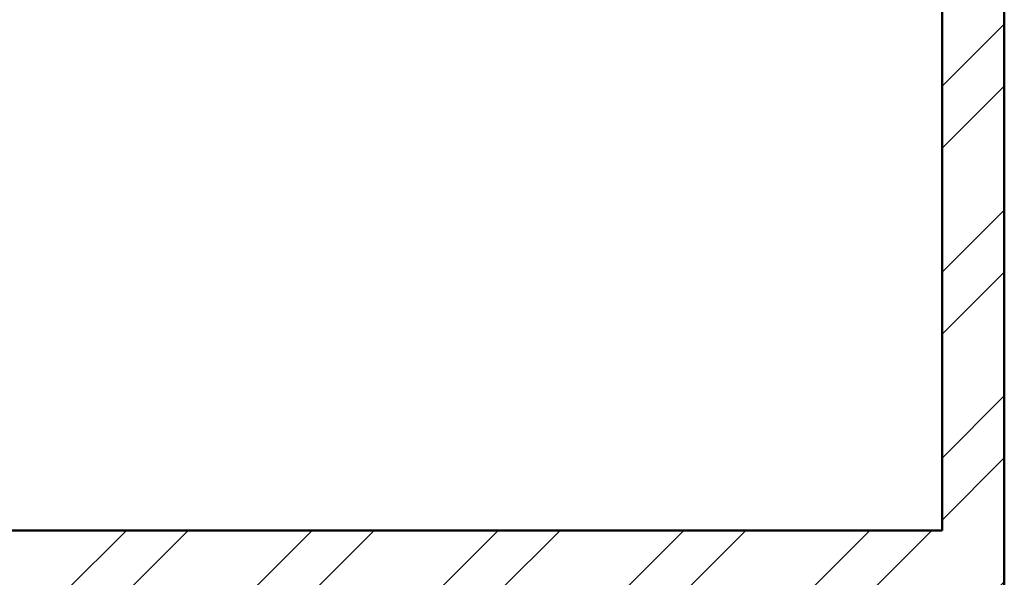
# Model space of a CAD drawing. Units: inches. Extents: x 1901 to 2863, y 888 to 2433.
# Tile 90 of 91: x 2682 to 2753, y 2080 to 2120. Entities that reach past the tile are written whole.
import ezdxf

# ---------------------------------------------------------------- set-up
doc = ezdxf.new("R2010")
doc.units = ezdxf.units.IN
doc.layers.add('A-WALL', color=7, linetype='Continuous', lineweight=50)
doc.layers.add('A-WALL-PATT', color=8, linetype='Continuous', lineweight=13)

msp = doc.modelspace()

# ---------------------------------------------------------------- hatches: boundary and pattern name
at = {"layer": 'A-WALL-PATT'}
h = msp.add_hatch(dxfattribs=at)
h.set_pattern_fill('ANSI32', color=256)
h.paths.add_polyline_path([(2192.501, 2274.134), (2141.264, 2274.134), (2141.264, 2269.634), (2192.501, 2269.634)])
h.paths.add_polyline_path([(2259.926, 2274.134), (2216.501, 2274.134), (2216.501, 2269.634), (2255.426, 2269.634), (2255.426, 2214.634), (2250.809, 2214.634), (2250.809, 2210.134), (2259.926, 2210.134), (2259.926, 2215.134), (2271.756, 2215.134), (2271.756, 2217.384), (2271.756, 2219.634), (2259.926, 2219.634)])
h.paths.add_polyline_path([(2171.426, 2269.634), (2166.926, 2269.634), (2166.926, 2219.634), (2121.238, 2219.634), (2121.238, 2215.134), (2166.926, 2215.134), (2166.926, 2083.134), (2161.807, 2083.134), (2161.807, 2078.634), (2171.426, 2078.634), (2176.996, 2078.634), (2176.996, 2080.884), (2176.996, 2083.134), (2171.426, 2083.134), (2171.426, 2210.134), (2230.912, 2210.134), (2230.912, 2212.384), (2230.912, 2214.634), (2171.426, 2214.634)])
h.paths.add_polyline_path([(2117.264, 2274.134), (2089.426, 2274.134), (2089.426, 2219.634), (2081.136, 2219.634), (2081.136, 2215.134), (2089.426, 2215.134), (2098.004, 2215.134), (2098.004, 2217.384), (2098.004, 2219.634), (2093.926, 2219.634), (2093.926, 2269.634), (2117.264, 2269.634), (2117.264, 2271.884)])
h.paths.add_polyline_path([(2343.426, 2219.634), (2329.295, 2219.634), (2329.295, 2215.134), (2338.926, 2215.134), (2338.926, 2184.739), (2343.426, 2184.739)])
h.paths.add_polyline_path([(2338.926, 2083.134), (2329.295, 2083.134), (2208.966, 2083.134), (2208.966, 2078.634), (2338.926, 2078.634)])
h.paths.add_polyline_path([(2343.426, 2136.739), (2338.926, 2136.739), (2338.926, 1872.634), (2343.426, 1872.634)])
h.paths.add_polyline_path([(2343.426, 1863.634), (2397.68, 1863.634), (2397.68, 1821.634), (2384.138, 1821.634), (2384.138, 1812.634), (2418.33, 1812.634), (2418.33, 1817.134), (2418.33, 1821.634), (2406.68, 1821.634), (2406.68, 1863.634), (2459.499, 1863.634), (2459.499, 1821.634), (2447.138, 1821.634), (2447.138, 1812.634), (2459.499, 1812.634), (2468.499, 1812.634), (2468.499, 1872.634), (2394.426, 1872.634), (2334.426, 1872.634), (2334.426, 1812.634), (2343.426, 1812.634), (2353.251, 1812.634), (2353.251, 1821.634), (2343.426, 1821.634)])
h.paths.add_polyline_path([(2510.014, 1872.634), (2468.499, 1872.634), (2468.499, 1868.134), (2510.014, 1868.134)])
h.paths.add_polyline_path([(2514.009, 1817.134), (2468.499, 1817.134), (2468.499, 1812.634), (2482.114, 1812.634), (2482.114, 1800.606), (2486.614, 1800.606), (2486.614, 1812.634), (2514.009, 1812.634)])
h.paths.add_polyline_path([(2299.247, 1814.884), (2299.247, 1817.134), (2295.926, 1817.134), (2295.926, 1854.169), (2293.676, 1854.169), (2291.426, 1854.169), (2291.426, 1817.134), (2266.109, 1817.134), (2266.109, 1812.634), (2299.247, 1812.634)])
h.paths.add_polyline_path([(2218.109, 1817.134), (2206.46, 1817.134), (2171.426, 1817.134), (2171.426, 1949.134), (2190.1, 1949.134), (2190.1, 1953.634), (2163.468, 1953.634), (2163.468, 1949.134), (2166.926, 1949.134), (2166.926, 1817.134), (2114.297, 1817.134), (2114.297, 1812.634), (2218.109, 1812.634)])
h.paths.add_polyline_path([(2029.426, 1970.922), (2024.926, 1970.922), (2024.926, 1912.717), (2029.426, 1912.717)])
h.paths.add_polyline_path([(2132.297, 1953.634), (2113.926, 1953.634), (2113.926, 1975.888), (2111.676, 1975.888), (2109.426, 1975.888), (2109.426, 1953.634), (2029.426, 1953.634), (2029.426, 1949.134), (2132.297, 1949.134)])
h.paths.add_polyline_path([(2029.426, 1853.606), (2029.31, 1853.606), (2029.31, 1853.606), (2029.426, 1853.606), (2029.426, 1864.717), (2024.926, 1864.717), (2024.926, 1812.634), (2066.297, 1812.634), (2066.297, 1814.884), (2066.297, 1817.134), (2029.426, 1817.134)])
h.paths.add_polyline_path([(2122.926, 2010.088), (2120.676, 2010.088), (2118.426, 2010.088), (2118.426, 2006.134), (2029.426, 2006.134), (2029.426, 2001.634), (2109.426, 2001.634), (2109.426, 1998.041), (2113.926, 1998.041), (2113.926, 2001.634), (2122.926, 2001.634)])
h.paths.add_polyline_path([(2029.426, 2031.376), (2024.926, 2031.376), (2024.926, 1994.922), (2027.176, 1994.922), (2029.426, 1994.922)])
h.paths.add_polyline_path([(2029.426, 2136.739), (2024.926, 2136.739), (2024.926, 2067.376), (2027.176, 2067.376), (2029.426, 2067.376)])
h.paths.add_polyline_path([(2125.618, 2083.134), (2029.426, 2083.134), (2029.426, 2078.634), (2118.426, 2078.634), (2118.426, 2030.715), (2122.926, 2030.715), (2122.926, 2078.634), (2125.618, 2078.634)])
h.paths.add_polyline_path([(2029.426, 2215.134), (2040.468, 2215.134), (2040.468, 2217.384), (2040.468, 2219.634), (2024.926, 2219.634), (2024.926, 2184.739), (2029.426, 2184.739), (2029.426, 2187.778)])
h.paths.add_polyline_path([(2686.426, 2274.134), (2659.284, 2274.134), (2659.284, 2269.634), (2681.926, 2269.634), (2681.926, 2219.634), (2676.816, 2219.634), (2676.816, 2215.134), (2681.926, 2215.134), (2697.011, 2215.134), (2697.011, 2217.384), (2697.011, 2219.634), (2686.426, 2219.634)])
h.paths.add_polyline_path([(2609.926, 2269.634), (2635.284, 2269.634), (2635.284, 2274.134), (2571.431, 2274.134), (2571.431, 2269.634), (2605.426, 2269.634), (2605.426, 2214.634), (2549.098, 2214.634), (2549.098, 2210.134), (2605.426, 2210.134), (2605.426, 2083.134), (2601.014, 2083.134), (2601.014, 2080.884), (2601.014, 2078.634), (2609.926, 2078.634), (2616.162, 2078.634), (2616.162, 2080.884), (2616.162, 2083.134), (2609.926, 2083.134), (2609.926, 2215.134), (2651.465, 2215.134), (2651.465, 2217.384), (2651.465, 2219.634), (2609.926, 2219.634)])
h.paths.add_polyline_path([(2521.426, 2269.634), (2547.431, 2269.634), (2547.431, 2271.884), (2547.431, 2274.134), (2516.926, 2274.134), (2516.926, 2219.634), (2506.41, 2219.634), (2506.41, 2215.134), (2516.926, 2215.134), (2516.926, 2210.134), (2525.402, 2210.134), (2525.402, 2212.384), (2525.402, 2214.634), (2521.426, 2214.634)])
h.paths.add_polyline_path([(2456.011, 2219.634), (2439.426, 2219.634), (2439.426, 2187.888), (2443.926, 2187.888), (2443.926, 2215.134), (2456.011, 2215.134)])
h.paths.add_polyline_path([(2752.926, 2219.634), (2739.485, 2219.634), (2739.485, 2215.134), (2748.426, 2215.134), (2748.426, 2187.888), (2752.926, 2187.888)])
h.paths.add_polyline_path([(2752.926, 2139.888), (2748.426, 2139.888), (2748.426, 2083.134), (2648.416, 2083.134), (2648.416, 2078.634), (2654.926, 2078.634), (2654.926, 2039.437), (2659.426, 2039.437), (2659.426, 2078.634), (2748.426, 2078.634), (2748.426, 2063.429), (2752.926, 2063.429)])
h.paths.add_polyline_path([(2752.926, 2010.634), (2659.426, 2010.634), (2659.426, 2015.652), (2654.926, 2015.652), (2654.926, 2010.634), (2605.426, 2010.634), (2605.426, 1920.967), (2609.926, 1920.967), (2609.926, 2006.134), (2748.426, 2006.134), (2748.426, 1982.466), (2752.926, 1982.466)])
h.paths.add_polyline_path([(2752.926, 2027.429), (2748.426, 2027.429), (2748.426, 2010.634), (2752.926, 2010.634)])
h.paths.add_polyline_path([(2748.426, 1886.134), (2609.926, 1886.134), (2609.926, 1889.719), (2605.426, 1889.719), (2605.426, 1861.262), (2609.926, 1861.262), (2609.926, 1881.634), (2748.426, 1881.634)])
h.paths.add_polyline_path([(2456.855, 2228.831), (2498.401, 2228.831), (2498.401, 2247.488), (2456.855, 2247.488)], flags=9)
h.paths.add_polyline_path([(2038.602, 2237.418), (2080.174, 2237.418), (2080.174, 2256.075), (2038.602, 2256.075)], flags=9)
h.paths.add_polyline_path([(2292.009, 1062.394), (2539.932, 1062.394), (2539.932, 1099.487), (2292.009, 1099.487)], flags=9)
h.paths.add_polyline_path([(2424.91, 1832.253), (2448.513, 1832.253), (2448.513, 1846.678), (2424.91, 1846.678)], flags=25)
h.paths.add_polyline_path([(2359.076, 1832.253), (2382.678, 1832.253), (2382.678, 1846.678), (2359.076, 1846.678)], flags=25)
h.paths.add_polyline_path([(2352.899, 1684.802), (2367.543, 1684.802), (2367.543, 1697.167), (2352.899, 1697.167)], flags=9)
h.paths.add_polyline_path([(2079.288, 1755.826), (2169.024, 1755.826), (2169.024, 1774.372), (2079.288, 1774.372)], flags=9)
h.paths.add_polyline_path([(2404.09, 1373.857), (2404.09, 1463.593), (2385.544, 1463.593), (2385.544, 1373.857)], flags=9)
h.paths.add_polyline_path([(2268.091, 2236.371), (2309.636, 2236.371), (2309.636, 2255.028), (2268.091, 2255.028)], flags=9)
h.paths.add_polyline_path([(2575.96, 1700.951), (2665.696, 1700.951), (2665.696, 1719.498), (2575.96, 1719.498)], flags=9)
h.paths.add_polyline_path([(2302.962, 1878.474), (2329.524, 1878.474), (2329.524, 1888.777), (2302.962, 1888.777)], flags=9)
h.paths.add_polyline_path([(2097.415, 2240.576), (2126.573, 2240.576), (2126.573, 2259.233), (2097.415, 2259.233)], flags=9)
h.paths.add_polyline_path([(2208.725, 2246.124), (2237.882, 2246.124), (2237.882, 2264.781), (2208.725, 2264.781)], flags=9)
h.paths.add_polyline_path([(2038.147, 1925.958), (2076.987, 1925.958), (2076.987, 1944.615), (2038.147, 1944.615)], flags=9)
h.paths.add_polyline_path([(2239.144, 1926.672), (2288.465, 1926.672), (2288.465, 1945.329), (2239.144, 1945.329)], flags=9)
h.paths.add_polyline_path([(2175.429, 2007.33), (2212.356, 2007.33), (2212.356, 2025.987), (2175.429, 2025.987)], flags=9)
h.paths.add_polyline_path([(2225.034, 2091.794), (2263.875, 2091.794), (2263.875, 2110.451), (2225.034, 2110.451)], flags=9)
h.paths.add_polyline_path([(2035.398, 2098.478), (2074.238, 2098.478), (2074.238, 2117.135), (2035.398, 2117.135)], flags=9)
h.paths.add_polyline_path([(2050.102, 2029.209), (2083.26, 2029.209), (2083.26, 2047.866), (2050.102, 2047.866)], flags=9)
h.paths.add_polyline_path([(2069.677, 1956.719), (2098.835, 1956.719), (2098.835, 1975.376), (2069.677, 1975.376)], flags=25)
h.paths.add_polyline_path([(2328.62, 1753.336), (2361.663, 1753.336), (2361.663, 1771.993), (2328.62, 1771.993)], flags=9)
h.paths.add_polyline_path([(2395.162, 2060.888), (2395.162, 2140.654), (2378.676, 2140.654), (2378.676, 2060.888)], flags=9)
h.paths.add_polyline_path([(2463.728, 2059.02), (2492.886, 2059.02), (2492.886, 2077.677), (2463.728, 2077.677)], flags=9)
h.paths.add_polyline_path([(2458.027, 2181.536), (2496.868, 2181.536), (2496.868, 2200.194), (2458.027, 2200.194)], flags=9)
h.paths.add_polyline_path([(2527.577, 2243.074), (2556.735, 2243.074), (2556.735, 2261.731), (2527.577, 2261.731)], flags=9)
h.paths.add_polyline_path([(2694.461, 2232.767), (2736.033, 2232.767), (2736.033, 2251.425), (2694.461, 2251.425)], flags=9)
h.paths.add_polyline_path([(2637.821, 2249.225), (2666.979, 2249.225), (2666.979, 2267.882), (2637.821, 2267.882)], flags=9)
h.paths.add_polyline_path([(2623.687, 2183.541), (2662.528, 2183.541), (2662.528, 2202.199), (2623.687, 2202.199)], flags=9)
h.paths.add_polyline_path([(2691.965, 2021.5), (2725.124, 2021.5), (2725.124, 2040.157), (2691.965, 2040.157)], flags=9)
h.paths.add_polyline_path([(2621.043, 1975.912), (2662.335, 1975.912), (2662.335, 1994.569), (2621.043, 1994.569)], flags=25)
h.paths.add_polyline_path([(2479.032, 1927.62), (2519.844, 1927.62), (2519.844, 1946.277), (2479.032, 1946.277)], flags=9)
h.paths.add_polyline_path([(2670.941, 1849.076), (2716.005, 1849.076), (2716.005, 1867.734), (2670.941, 1867.734)], flags=9)
h.paths.add_polyline_path([(2523.613, 1782.956), (2550.175, 1782.956), (2550.175, 1793.26), (2523.613, 1793.26)], flags=9)
h.paths.add_polyline_path([(2450.841, 1207.331), (2492.386, 1207.331), (2492.386, 1225.989), (2450.841, 1225.989)], flags=9)
h.paths.add_polyline_path([(2527.751, 1203.841), (2556.908, 1203.841), (2556.908, 1222.499), (2527.751, 1222.499)], flags=9)
h.paths.add_polyline_path([(2639.111, 1207.2), (2668.268, 1207.2), (2668.268, 1225.857), (2639.111, 1225.857)], flags=9)
h.paths.add_polyline_path([(2692.594, 1218.965), (2734.167, 1218.965), (2734.167, 1237.623), (2692.594, 1237.623)], flags=9)
h.paths.add_polyline_path([(2669.266, 1366.329), (2708.106, 1366.329), (2708.106, 1384.987), (2669.266, 1384.987)], flags=9)
h.paths.add_polyline_path([(2463.313, 1358.031), (2502.153, 1358.031), (2502.153, 1376.688), (2463.313, 1376.688)], flags=9)
h.paths.add_polyline_path([(2494.725, 1449.963), (2531.652, 1449.963), (2531.652, 1468.62), (2494.725, 1468.62)], flags=9)
h.paths.add_polyline_path([(2675.565, 1422.157), (2708.724, 1422.157), (2708.724, 1440.815), (2675.565, 1440.815)], flags=9)
h.paths.add_polyline_path([(2685.634, 1493.891), (2714.792, 1493.891), (2714.792, 1512.548), (2685.634, 1512.548)], flags=9)
h.paths.add_polyline_path([(2686.805, 1529.913), (2725.645, 1529.913), (2725.645, 1548.57), (2686.805, 1548.57)], flags=9)
h.paths.add_polyline_path([(2503.651, 1537.991), (2552.972, 1537.991), (2552.972, 1556.648), (2503.651, 1556.648)], flags=9)
h.paths.add_polyline_path([(2291.713, 1643.504), (2318.275, 1643.504), (2318.275, 1653.807), (2291.713, 1653.807)], flags=9)
h.paths.add_polyline_path([(2450.626, 1610.52), (2477.189, 1610.52), (2477.189, 1620.824), (2450.626, 1620.824)], flags=9)
h.paths.add_polyline_path([(2359.985, 1551.814), (2422.253, 1551.814), (2422.253, 1562.117), (2359.985, 1562.117)], flags=9)
h.paths.add_polyline_path([(2280.106, 1249.006), (2321.651, 1249.006), (2321.651, 1267.663), (2280.106, 1267.663)], flags=9)
h.paths.add_polyline_path([(2164.057, 1274.232), (2193.215, 1274.232), (2193.215, 1292.889), (2164.057, 1292.889)], flags=9)
h.paths.add_polyline_path([(2118.21, 1277.694), (2151.252, 1277.694), (2151.252, 1296.351), (2118.21, 1296.351)], flags=9)
h.paths.add_polyline_path([(2031.946, 1268.529), (2073.519, 1268.529), (2073.519, 1287.187), (2031.946, 1287.187)], flags=9)
h.paths.add_polyline_path([(2050.199, 1409.079), (2089.04, 1409.079), (2089.04, 1427.736), (2050.199, 1427.736)], flags=9)
h.paths.add_polyline_path([(2243.743, 1421.032), (2282.584, 1421.032), (2282.584, 1439.689), (2243.743, 1439.689)], flags=9)
h.paths.add_polyline_path([(2190.746, 1509.769), (2231.558, 1509.769), (2231.558, 1528.426), (2190.746, 1528.426)], flags=9)
h.paths.add_polyline_path([(2058.392, 1475.415), (2091.55, 1475.415), (2091.55, 1494.073), (2058.392, 1494.073)], flags=9)
h.paths.add_polyline_path([(2062.447, 1553.09), (2091.605, 1553.09), (2091.605, 1571.747), (2062.447, 1571.747)], flags=9)
h.paths.add_polyline_path([(2219.524, 1590.365), (2266.147, 1590.365), (2266.147, 1609.022), (2219.524, 1609.022)], flags=9)
h.paths.add_polyline_path([(2041.072, 1584.188), (2079.912, 1584.188), (2079.912, 1602.845), (2041.072, 1602.845)], flags=9)

# ---------------------------------------------------------------- linework, layer by layer
at = {"layer": 'A-WALL'}
for p, q in [((2752.926, 2219.634), (2752.926, 1812.634)), ((2748.426, 2215.134), (2748.426, 2083.134)), ((2646.874, 2083.134), (2748.426, 2083.134)), ((2681.926, 2083.134), (2697.011, 2083.134))]:
    msp.add_line(p, q, dxfattribs=at)

doc.saveas('drawing.dxf')
